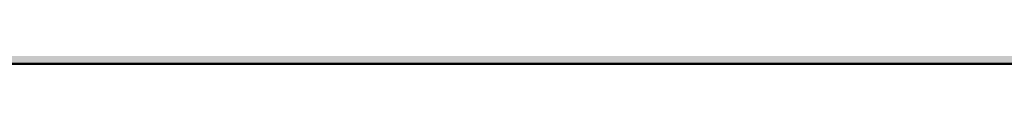
# Model space of a CAD drawing. Units: millimetres. Extents: x 0 to 2267, y 0 to 1823.
# Tile 188 of 256: x 1838.83 to 1841.442, y 1127.417 to 1127.417. Entities that reach past the tile are written whole.
import ezdxf

# ---------------------------------------------------------------- set-up
doc = ezdxf.new("R2010")
doc.units = ezdxf.units.MM
doc.header["$MEASUREMENT"] = 0
for name, color, linetype, lineweight in [('M-DIMS', 2, 'Continuous', 25), ('M-HATC', 252, 'Continuous', 18), ('M-OUTL', 7, 'Continuous', 50)]:
    doc.layers.add(name, color=color, linetype=linetype, lineweight=lineweight)
doc.styles.get("Standard").update_dxf_attribs({"font": 'arial.ttf'})
doc.dimstyles.get("Standard").update_dxf_attribs({"dimtxt": 7, "dimasz": 4, "dimexe": 0.18, "dimexo": 0.0625, "dimgap": 0.09, "dimtad": 0, "dimdec": 0, "dimzin": 0, "dimdsep": 46, "dimtxsty": 'Standard', "dimcen": 0.09, "dimadec": 0, "dimazin": 0, "dimtfac": 1, "dimtdec": 0, "dimtofl": 0, "dimtmove": 0, "dimatfit": 3, "dimfxl": 1, "dimtolj": 1, "dimtzin": 0, "dimarcsym": 0})

# ---------------------------------------------------------------- blocks, each defined once
blk = doc.blocks.new('*D1')
at = {"layer": 'Defpoints', "color": 0, "transparency": 16777216}
for p in [(1593.4289, 1127.4171), (1843.4289, 1127.4171), (1843.4289, 955.6278)]:
    blk.add_point(p, dxfattribs=at)
at = {"layer": 'M-DIMS', "color": 0, "lineweight": -2, "transparency": 16777216}
for p, q in [((1593.4289, 1127.3546), (1593.4289, 955.4478)), ((1843.4289, 1127.3546), (1843.4289, 955.4478)), ((1597.4289, 955.6278), (1710.5582, 955.6278)), ((1839.4289, 955.6278), (1726.2996, 955.6278))]:
    blk.add_line(p, q, dxfattribs=at)
at = {"layer": 'M-DIMS', "color": 0, "transparency": 16777216}
for points in [[(1597.4289, 956.2944), (1597.4289, 954.9611), (1593.4289, 955.6278)], [(1839.4289, 956.2944), (1839.4289, 954.9611), (1843.4289, 955.6278)]]:
    blk.add_solid(points, dxfattribs=at)
at = {"layer": 'M-DIMS', "color": 0, "transparency": 16777216, "insert": (1718.4289, 955.6278), "char_height": 7, "attachment_point": 5}
blk.add_mtext('\\A1;250', dxfattribs=at)

msp = doc.modelspace()

# ---------------------------------------------------------------- hatches: boundary and pattern name
at = {"layer": 'M-HATC'}
h = msp.add_hatch(color=256, dxfattribs=at)
h.dxf.hatch_style = 1
h.paths.add_polyline_path([(2042.8886, 1580.1796), (2055.771, 1593.062), (1381.0868, 1593.062), (1393.9692, 1580.1796), (1374.086, 1560.2964), (2062.7718, 1560.2964)])
h.paths.add_polyline_path([(1843.4289, 1201.3297), (1843.4289, 1227.2475), (1593.4289, 1227.2475), (1593.4289, 1201.3297, -0.228274), (1574.5989, 1162.2346), (1530.9289, 1127.4171), (1905.9289, 1127.4171), (1862.2589, 1162.2346, -0.228274)])

# ---------------------------------------------------------------- linework, layer by layer
at = {"layer": 'M-OUTL'}
msp.add_line((1530.9289, 1127.4171), (1905.9289, 1127.4171), dxfattribs=at)

# ---------------------------------------------------------------- dimensions: what is measured, and where the dimension line sits
at = {"layer": 'M-DIMS'}
dim = msp.add_linear_dim(base=(1843.4289, 955.6278), p1=(1593.4289, 1127.4171), p2=(1843.4289, 1127.4171), dimstyle='Standard', override={"dimclrd": 0, "dimclre": 0, "dimclrt": 0}, dxfattribs=at)
dim.commit()
dim.dimension.update_dxf_attribs({"geometry": '*D1', "text_midpoint": (1718.4289, 955.6278)})

doc.saveas('drawing.dxf')
